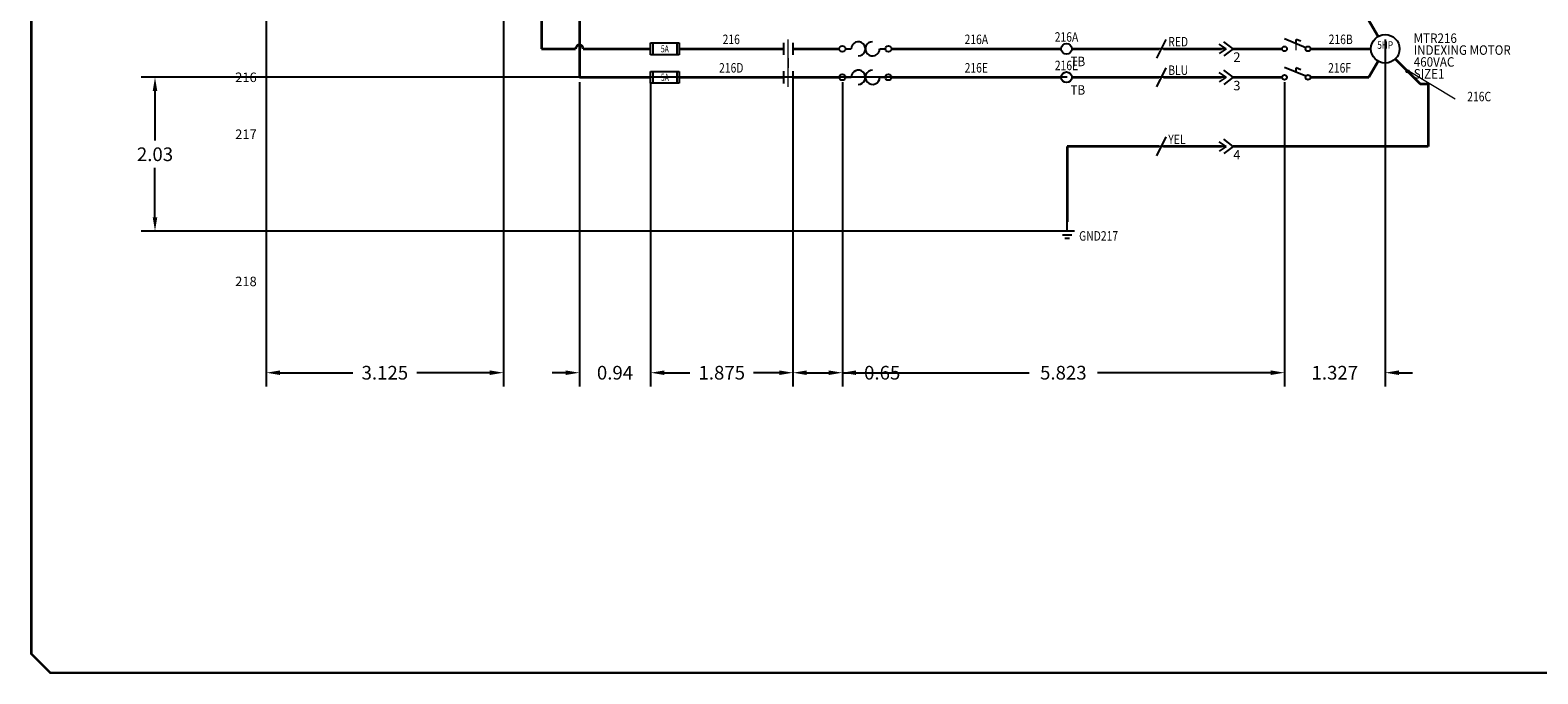
# Model space of a CAD drawing. Extents: x 0 to 33.5, y 0 to 22.4.
# Tile 1 of 8: x 0 to 19.9, y 0 to 8.5. Entities that reach past the tile are written whole.
import ezdxf
from ezdxf.enums import TextEntityAlignment as Align

# ---------------------------------------------------------------- set-up
doc = ezdxf.new("R2010")
doc.units = 0
doc.header["$MEASUREMENT"] = 0
for name, color, linetype, lineweight in [('A-ANNO-DIMS', 2, 'Continuous', 18), ('E-ANNO-TEXT', 3, 'Continuous', 18), ('LINK', 9, 'Continuous', 18), ('MISC', 7, 'Continuous', 13), ('SYMS', 7, 'Continuous', 25), ('TITLE', 7, 'Continuous', 35), ('WIRENO', 72, 'Continuous', 18), ('WIRES', 7, 'Continuous', 35)]:
    doc.layers.add(name, color=color, linetype=linetype, lineweight=lineweight)
for name, color, linetype in [('DESC', 150, 'Continuous'), ('TAGS', 150, 'Continuous'), ('TERMS', 123, 'Continuous'), ('WIREREF', 52, 'Continuous')]:
    doc.layers.add(name, color=color, linetype=linetype)
doc.styles.add('ITALIC', font='ITALIC')
doc.styles.add('SIMPLEX', font='SIMPLEX')
doc.styles.add('WD', font='romans.shx')
doc.dimstyles.get("Standard").update_dxf_attribs({"dimtxt": 0.18, "dimasz": 0.18, "dimexe": 0.18, "dimexo": 0.0625, "dimgap": 0.09, "dimtad": 0, "dimtih": 1, "dimtoh": 1, "dimdec": 4, "dimzin": 0, "dimdsep": 46, "dimtxsty": 'Standard', "dimcen": 0.09, "dimadec": 0, "dimazin": 0, "dimtfac": 1, "dimtdec": 4, "dimtofl": 0, "dimtmove": 0, "dimatfit": 3, "dimfxl": 1, "dimtolj": 1, "dimtzin": 0, "dimarcsym": 0})

# ---------------------------------------------------------------- blocks, each defined once
blk = doc.blocks.new('NO_NUM_acade_title')
at = {"layer": 'TITLE', "const_width": 0.0312}
blk.add_lwpolyline([(30.594, 0.281), (30.594, 22.177), (30.344, 22.427), (0.281, 22.427), (0.031, 22.177), (0.031, 0.281), (0.281, 0.031), (30.344, 0.031)], close=True, dxfattribs=at)
at = {"layer": 'TITLE', "style": 'ITALIC'}
for tag, height, p in [('TITLE#1', 0.125, (32.156, 3.406)), ('TITLE#2', 0.125, (32.156, 3.204)), ('TITLE#3', 0.125, (32.156, 3.001)), ('TITLE#4', 0.125, (32.156, 2.799)), ('DWG#', 0.2, (32.156, 0.826))]:
    blk.add_attdef(tag, text='', height=height, dxfattribs=at).set_placement(p, align=Align.CENTER)
at = {"layer": 'TITLE', "style": 'SIMPLEX'}
blk.add_attdef('CAD#', (30.826, 1.958), '', height=0.0938, rotation=90, dxfattribs=at)
at = {"layer": 'TITLE'}
for tag, p, height, style in [('JOB#', (31.464, 1.644), 0.0938, 'SIMPLEX'), ('SCALE', (31.353, 1.344), 0.0938, 'SIMPLEX'), ('DATE', (32.408, 1.344), 0.0938, 'SIMPLEX'), ('SHTS', (32.532, 0.25), 0.2, 'ITALIC')]:
    blk.add_attdef(tag, p, '', height=height, dxfattribs=dict(at, style=style))
at = {"layer": 'TITLE', "style": 'ITALIC'}
blk.add_attdef('SH#', text='', height=0.2, dxfattribs=at).set_placement((31.881, 0.25), align=Align.RIGHT)
at = {"layer": 'TITLE', "flags": 9}
blk.add_attdef('WD_TB', (31.219, 0.031), '', height=0.125, dxfattribs=at)
blk = doc.blocks.new('HFU1')
for p, q in [((-0.188, -0.078), (-0.188, 0.078)), ((-0.188, 0.078), (0.188, 0.078)), ((-0.156, 0.078), (-0.156, -0.078)), ((0.156, 0.078), (0.156, -0.078)), ((0.188, 0.078), (0.188, -0.078)), ((0.188, -0.078), (-0.188, -0.078))]:
    blk.add_line(p, q)
at = {"style": 'WD', "width": 0.7}
for tag, p in [('INST', (0, 0.422)), ('TAG1', (0, 0.125)), ('LOC', (0, 0.266))]:
    blk.add_attdef(tag, text='', height=0.125, dxfattribs=at).set_placement(p, align=Align.CENTER)
at = {"style": 'WD', "flags": 9}
for tag, p in [('ASSYCODE', (0.157, 0.251)), ('MFG', (0.156, 0.083)), ('CAT', (0.156, 0.102))]:
    blk.add_attdef(tag, text='', height=0.01, dxfattribs=at).set_placement(p, align=Align.CENTER)
at = {"style": 'WD'}
for tag, p, height, flags in [('X4TERM01', (-0.188, 0), 0.0109, 1), ('FAMILY', (0.129, 0.108), 0.01, 9), ('X1TERM02', (0.188, 0), 0.0109, 1)]:
    blk.add_attdef(tag, p, '', height=height, dxfattribs=dict(at, flags=flags))
at = {"style": 'WD', "width": 0.7}
blk.add_attdef('RATING1', text='', height=0.0938, dxfattribs=at).set_placement((0, 0), align=Align.MIDDLE_CENTER)
at = {"style": 'WD'}
for tag, p in [('X2LINK', (0, 0.109)), ('X8LINK', (0, -0.109))]:
    blk.add_attdef(tag, p, '', height=0.01, dxfattribs=at)
at = {"style": 'WD', "width": 0.7, "flags": 8}
blk.add_attdef('TERM01', text='', height=0.1, dxfattribs=at).set_placement((-0.25, -0.016), align=Align.TOP_RIGHT)
at = {"style": 'WD', "width": 0.7}
for tag, p in [('DESC1', (0.047, -0.234)), ('DESC2', (0.047, -0.391)), ('DESC3', (0.047, -0.547))]:
    blk.add_attdef(tag, text='', height=0.125, dxfattribs=at).set_placement(p, align=Align.MIDDLE_LEFT)
at = {"style": 'WD', "width": 0.7, "flags": 8}
blk.add_attdef('TERM02', text='', height=0.1, dxfattribs=at).set_placement((0.25, -0.016), align=Align.TOP_LEFT)
blk = doc.blocks.new('HCR21')
for p, q in [((-0.062, 0.08), (-0.062, -0.08)), ((0.062, 0.08), (0.062, -0.08))]:
    blk.add_line(p, q)
at = {"style": 'WD'}
for tag, width, p in [('INST', 0.7, (0, 0.451)), ('LOC', 0.7, (0, 0.281)), ('TAG2', 0.9, (0, 0.125)), ('XREF', 0.7, (0, -0.297)), ('DESC1', 0.7, (0, -0.449)), ('DESC2', 0.7, (0, -0.597)), ('DESC3', 0.7, (0, -0.744))]:
    blk.add_attdef(tag, text='', height=0.125, dxfattribs=dict(at, width=width)).set_placement(p, align=Align.CENTER)
for tag, p, height, flags in [('X4TERM01', (-0.062, 0), 0.0125, 1), ('X1TERM02', (0.062, 0), 0.0125, 1), ('CONTACT', (0.097, 0.036), 0.01, 1), ('FAMILY', (0.097, 0.053), 0.01, 9)]:
    blk.add_attdef(tag, p, '', height=height, dxfattribs=dict(at, flags=flags))
for tag, p in [('X2LINK', (0, 0.125)), ('X8LINK', (0, -0.125))]:
    blk.add_attdef(tag, p, '', height=0.01, dxfattribs=at)
at = {"style": 'WD', "flags": 8}
blk.add_attdef('TERM01', text='', height=0.125, dxfattribs=at).set_placement((-0.125, -0.016), align=Align.TOP_RIGHT)
blk.add_attdef('TERM02', text='', height=0.125, dxfattribs=at).set_placement((0.125, -0.016), align=Align.TOP_LEFT)
blk = doc.blocks.new('HOL1')
for p, q in [((-0.264, 0), (-0.188, 0)), ((0.188, 0), (0.264, 0))]:
    blk.add_line(p, q)
for centre in [(-0.304, 0), (0.304, 0)]:
    blk.add_circle(centre, 0.04)
for centre, start, end in [((-0.094, 0), 270.001, 180.002), ((0.094, 0), 90, 0.001)]:
    blk.add_arc(centre, 0.0938, start, end)
at = {"style": 'WD', "width": 0.7}
for tag, p in [('INST', (0, 0.795)), ('DESC1', (0, 0.469)), ('LOC', (0, 0.625)), ('DESC2', (0, 0.312)), ('RATING1', (0, -0.266))]:
    blk.add_attdef(tag, text='', height=0.125, dxfattribs=at).set_placement(p, align=Align.CENTER)
at = {"style": 'WD'}
blk.add_attdef('TAG1', text='', height=0.125, dxfattribs=at).set_placement((0, 0.156), align=Align.CENTER)
for tag, p, height, flags in [('X4TERM01', (-0.344, 0), 0.0125, 1), ('FAMILY', (0.205, 0.152), 0.01, 9), ('X1TERM02', (0.344, 0), 0.0125, 1)]:
    blk.add_attdef(tag, p, '', height=height, dxfattribs=dict(at, flags=flags))
for tag, p in [('X2LINK', (0, 0.125)), ('X8LINK', (0, -0.125))]:
    blk.add_attdef(tag, p, '', height=0.01, dxfattribs=at)
at = {"style": 'WD', "flags": 9}
for tag, p in [('ASSYCODE', (0.219, 0.062)), ('MFG', (0.228, 0.089)), ('CAT', (0.23, 0.108))]:
    blk.add_attdef(tag, text='', height=0.01, dxfattribs=at).set_placement(p, align=Align.CENTER)
at = {"style": 'WD', "flags": 8}
blk.add_attdef('TERM01', text='', height=0.125, dxfattribs=at).set_placement((-0.406, -0.031), align=Align.TOP_RIGHT)
blk.add_attdef('TERM02', text='', height=0.125, dxfattribs=at).set_placement((0.406, -0.031), align=Align.TOP_LEFT)
blk = doc.blocks.new('HT0W02')
blk.add_circle((0, 0), 0.0699)
at = {"style": 'WD'}
for tag, p, width in [('INST', (0.062, 0.42), 0.7), ('LOC', (0.062, 0.25), 0.7), ('DESC1', (0.053, -0.385), 0.8)]:
    blk.add_attdef(tag, p, '', height=0.125, dxfattribs=dict(at, width=width))
at = {"style": 'WD', "width": 0.8, "flags": 8}
blk.add_attdef('WIRENO', text='', height=0.125, dxfattribs=at).set_placement((0, 0.094), align=Align.CENTER)
at = {"style": 'WD', "flags": 1}
for tag, p, height in [('X4TERM01', (-0.07, 0), 0.0125), ('X4TERMDESC01', (-0.055, -0.023), 0.025), ('X2TERMDESC01', (-0.006, 0.029), 0.025), ('X2TERM01', (0, 0.07), 0.0125), ('STRIPSEQ', (0, 0), 0.00125), ('X1TERMDESC01', (0.039, -0.003), 0.025), ('X1TERM01', (0.07, 0), 0.0125), ('LINKTERM', (0, -0.002), 0.00125), ('X8TERM01', (0, -0.07), 0.0125), ('X8TERMDESC01', (0, -0.054), 0.025)]:
    blk.add_attdef(tag, p, '', height=height, dxfattribs=at)
at = {"style": 'WD'}
for tag, p, height, width, flags in [('TAGSTRIP', (0.053, -0.229), 0.125, 0.9, 8), ('ASSYCODE', (0.062, -0.281), 0.01, 0.7, 1), ('CAT', (0.213, -0.406), 0.109, 0.8, 1), ('DESC2', (0.053, -0.541), 0.125, 0.8, 8), ('DESC3', (0.053, -0.698), 0.125, 0.8, 8)]:
    blk.add_attdef(tag, p, '', height=height, dxfattribs=dict(at, width=width, flags=flags))
at = {"style": 'WD', "width": 0.8, "flags": 1}
blk.add_attdef('MFG', text='', height=0.109, dxfattribs=at).set_placement((0.088, -0.406), align=Align.RIGHT)
blk = doc.blocks.new('HDS11')
for p, q in [((0.126, 0.013), (-0.156, 0.13)), ((0, 0.065), (0, 0.125)), ((0.062, 0.099), (0, 0.125))]:
    blk.add_line(p, q)
for centre in [(-0.155, 0), (0.155, 0)]:
    blk.add_circle(centre, 0.0322)
at = {"style": 'WD', "width": 0.7}
for tag, p in [('INST', (0, 0.625)), ('LOC', (0, 0.469)), ('RATING1', (0, 0.156)), ('XREF', (0, -0.236)), ('DESC1', (0, -0.406)), ('DESC2', (0, -0.562))]:
    blk.add_attdef(tag, text='', height=0.125, dxfattribs=at).set_placement(p, align=Align.CENTER)
at = {"style": 'WD'}
blk.add_attdef('TAG1', text='', height=0.125, dxfattribs=at).set_placement((0, 0.312), align=Align.CENTER)
for tag, p in [('X2LINK', (0, 0.438)), ('X8LINK', (0, -0.016))]:
    blk.add_attdef(tag, p, '', height=0.01, dxfattribs=at)
for tag, p, height, flags in [('X4TERM01', (-0.188, 0), 0.0125, 1), ('X1TERM02', (0.188, 0), 0.0125, 1), ('CONTACT', (0.206, 0.04), 0.01, 9), ('FAMILY', (0.206, 0.131), 0.01, 9)]:
    blk.add_attdef(tag, p, '', height=height, dxfattribs=dict(at, flags=flags))
at = {"style": 'WD', "flags": 9}
for tag, p in [('ASSYCODE', (0.219, 0.062)), ('MFG', (0.228, 0.089)), ('CAT', (0.23, 0.108))]:
    blk.add_attdef(tag, text='', height=0.01, dxfattribs=at).set_placement(p, align=Align.CENTER)
at = {"style": 'WD', "flags": 8}
blk.add_attdef('TERM01', text='', height=0.125, dxfattribs=at).set_placement((-0.25, -0.031), align=Align.TOP_RIGHT)
blk.add_attdef('TERM02', text='', height=0.125, dxfattribs=at).set_placement((0.25, -0.031), align=Align.TOP_LEFT)
blk = doc.blocks.new('HMO13')
blk.add_circle((0, 0), 0.188)
at = {"style": 'WD'}
for tag, p, width in [('INST', (0.381, 0.403), 0.7), ('TAG1', (0.375, 0.077), 0.9), ('LOC', (0.381, 0.234), 0.7), ('DESC1', (0.376, -0.079), 0.9), ('DESC2', (0.376, -0.235), 0.9), ('DESC3', (0.376, -0.391), 0.9), ('RATING3', (0.375, -0.548), 0.8), ('RATING4', (0.375, -0.704), 0.8), ('WDTAGALT', (0.375, -0.875), 0.7)]:
    blk.add_attdef(tag, p, '', height=0.125, dxfattribs=dict(at, width=width))
at = {"style": 'WD', "width": 0.8}
blk.add_attdef('RATING1', text='', height=0.1, dxfattribs=at).set_placement((0, 0), align=Align.CENTER)
at = {"style": 'WD', "flags": 1}
for tag, p in [('X4TERM02', (-0.188, 0)), ('X0TERM01', (-0.094, 0.162)), ('X0TERM03', (-0.094, -0.162)), ('X0TERM04', (0.133, -0.133))]:
    blk.add_attdef(tag, p, '', height=0.0125, dxfattribs=at)
at = {"style": 'WD', "flags": 9}
for tag, p in [('ASSYCODE', (0, 0.125)), ('FAMILY', (-0.005, 0.17))]:
    blk.add_attdef(tag, text='', height=0.01, dxfattribs=at).set_placement(p, align=Align.CENTER)
at = {"style": 'WD', "flags": 1}
for tag, p in [('MFG', (0, 0.14)), ('CAT', (0, 0.159))]:
    blk.add_attdef(tag, text='', height=0.01, dxfattribs=at).set_placement(p, align=Align.MIDDLE)
at = {"style": 'WD', "width": 0.8}
blk.add_attdef('RATING2', text='', height=0.1, dxfattribs=at).set_placement((0, -0.031), align=Align.TOP_CENTER)
blk = doc.blocks.new('VGND2')
for p, q in [((0, -0.125), (0, 0)), ((0.09375, -0.125), (-0.09375, -0.125)), ((-0.0625, -0.171875), (0.0625, -0.171875)), ((-0.03125, -0.21875), (0.03125, -0.21875))]:
    blk.add_line(p, q)
at = {"style": 'WD', "flags": 1}
for tag in ['ASSYCODE', 'X2TERM01', 'CAT', 'MFG', 'FAMILY']:
    blk.add_attdef(tag, (0, 0), '', height=0.01, dxfattribs=at)
at = {"style": 'WD', "width": 0.8}
for tag, p in [('INST', (0.15625, 0.125)), ('LOC', (0.15625, -0.03125)), ('TAG1', (0.15625, -0.1875)), ('DESC1', (0.15625, -0.34375)), ('DESC2', (0.15625, -0.5))]:
    blk.add_attdef(tag, text='', height=0.125, dxfattribs=at).set_placement(p, align=Align.MIDDLE_LEFT)
blk = doc.blocks.new('HCN2PJ')
for p, q in [((-0.031, 0), (-0.125, 0.062)), ((-0.031, 0), (-0.125, -0.062)), ((-0.031, 0), (-0.094, 0)), ((0.062, 0), (-0.062, 0.094)), ((0.062, 0), (-0.062, -0.094))]:
    blk.add_line(p, q)
at = {"style": 'WD', "width": 0.7}
for tag, p in [('DESC1', (-0.031, 0.406)), ('DESC2', (-0.031, 0.25))]:
    blk.add_attdef(tag, text='', height=0.125, dxfattribs=at).set_placement(p, align=Align.RIGHT)
for tag, p in [('INST', (0.094, 0.406)), ('LOC', (0.094, 0.25))]:
    blk.add_attdef(tag, p, '', height=0.125, dxfattribs=at)
at = {"style": 'WD'}
for tag, p, height in [('TAG2', (0.094, 0.094), 0.125), ('X2LINK', (-0.062, 0.125), 0.01), ('X8LINK', (-0.062, -0.125), 0.01)]:
    blk.add_attdef(tag, p, '', height=height, dxfattribs=at)
for tag, p, height, flags in [('X4TERMDESC01', (-0.113, 0.019), 0.01, 1), ('X4TERM01', (-0.094, 0), 0.0125, 1), ('FAMILY', (0.048, 0.121), 0.01, 9), ('X1TERM02', (0.062, 0), 0.0125, 1), ('X1TERMDESC02', (0.067, 0.014), 0.01, 1)]:
    blk.add_attdef(tag, p, '', height=height, dxfattribs=dict(at, flags=flags))
at = {"style": 'WD', "flags": 8}
blk.add_attdef('TERM01', text='', height=0.125, dxfattribs=at).set_placement((-0.156, -0.047), align=Align.TOP_RIGHT)
blk.add_attdef('TERM02', text='', height=0.125, dxfattribs=at).set_placement((0.062, -0.047), align=Align.TOP_LEFT)
blk = doc.blocks.new('HW02')
for p, q in [((0.062, 0.125), (-0.062, -0.125)), ((0.031, 0), (-0.031, 0))]:
    blk.add_line(p, q)
at = {"style": 'WD', "width": 0.7, "flags": 1}
for tag, p in [('INST', (0, 0.357)), ('LOC', (0, 0.188)), ('XREF', (0, -0.3)), ('DESC1', (0, -0.456)), ('DESC2', (0, -0.613))]:
    blk.add_attdef(tag, text='', height=0.125, dxfattribs=at).set_placement(p, align=Align.CENTER)
at = {"style": 'WD', "width": 0.8}
blk.add_attdef('TAG2', text='', height=0.125, dxfattribs=at).set_placement((-0.031, 0.031), align=Align.RIGHT)
at = {"style": 'WD', "flags": 1}
for tag, p in [('X4TERM01', (-0.031, 0)), ('X1TERM01', (0.031, 0))]:
    blk.add_attdef(tag, p, '', height=0.0125, dxfattribs=at)
at = {"style": 'WD'}
for tag, p in [('X2LINK', (0, 0.125)), ('X8LINK', (0, -0.125))]:
    blk.add_attdef(tag, p, '', height=0.01, dxfattribs=at)
at = {"style": 'WD', "flags": 9}
blk.add_attdef('FAMILY', text='', height=0.01, dxfattribs=at).set_placement((0.023, 0.118), align=Align.CENTER)
at = {"style": 'WD', "width": 0.8}
blk.add_attdef('RATING1', (0.094, 0.031), '', height=0.125, dxfattribs=at)
blk = doc.blocks.new('WD_WNH')
at = {"style": 'WD', "width": 0.8}
blk.add_attdef('WIRENO', text='', height=0.125, dxfattribs=at).set_placement((0, 0.062), align=Align.CENTER)
at = {"style": 'WD', "flags": 1}
for tag, p in [('W01USER', (0, 0.078)), ('W02USER', (0, 0.07)), ('W03USER', (0, 0.062)), ('W04USER', (0, 0.055)), ('W05USER', (0, 0.047)), ('W06USER', (0, 0.039)), ('W07USER', (0, 0.031)), ('W08USER', (0, 0.023)), ('W09USER', (0, 0.016)), ('W10USER', (0, 0.008))]:
    blk.add_attdef(tag, text='', height=0.005, dxfattribs=at).set_placement(p, align=Align.CENTER)
blk = doc.blocks.new('*D36')
at = {"layer": 'A-ANNO-DIMS', "color": 0, "lineweight": -2, "transparency": 16777216}
for p, q in [((3.125, 17.5625), (3.125, 3.802917)), ((6.25, 17.5625), (6.25, 3.802917)), ((3.305, 3.982917), (4.2675, 3.982917)), ((6.07, 3.982917), (5.1075, 3.982917))]:
    blk.add_line(p, q, dxfattribs=at)
at = {"layer": 'A-ANNO-DIMS', "color": 0, "transparency": 16777216}
for points in [[(3.305, 4.012917), (3.305, 3.952917), (3.125, 3.982917)], [(6.07, 4.012917), (6.07, 3.952917), (6.25, 3.982917)]]:
    blk.add_solid(points, dxfattribs=at)
at = {"layer": 'Defpoints', "color": 0, "transparency": 16777216}
for p in [(3.125, 17.625), (6.25, 17.625), (6.25, 3.982917)]:
    blk.add_point(p, dxfattribs=at)
at = {"layer": 'A-ANNO-DIMS', "color": 0, "transparency": 16777216, "insert": (4.6875, 3.982917), "char_height": 0.18, "attachment_point": 5}
blk.add_mtext('\\A1;3.125', dxfattribs=at)
blk = doc.blocks.new('*D41')
at = {"layer": 'A-ANNO-DIMS', "color": 0, "lineweight": -2, "transparency": 16777216}
for p, q in [((7.25, 7.8125), (7.25, 3.802917)), ((8.1875, 7.8125), (8.1875, 3.802917)), ((7.07, 3.982917), (6.89, 3.982917)), ((8.3675, 3.982917), (8.5475, 3.982917))]:
    blk.add_line(p, q, dxfattribs=at)
at = {"layer": 'A-ANNO-DIMS', "color": 0, "transparency": 16777216}
for points in [[(7.07, 4.012917), (7.07, 3.952917), (7.25, 3.982917)], [(8.3675, 4.012917), (8.3675, 3.952917), (8.1875, 3.982917)]]:
    blk.add_solid(points, dxfattribs=at)
at = {"layer": 'Defpoints', "color": 0, "transparency": 16777216}
for p in [(7.25, 7.875), (8.1875, 7.875), (8.1875, 3.982917)]:
    blk.add_point(p, dxfattribs=at)
at = {"layer": 'A-ANNO-DIMS', "color": 0, "transparency": 16777216, "insert": (7.71875, 3.982917), "char_height": 0.18, "attachment_point": 5}
blk.add_mtext('\\A1;0.94', dxfattribs=at)
blk = doc.blocks.new('*D42')
at = {"layer": 'A-ANNO-DIMS', "color": 0, "lineweight": -2, "transparency": 16777216}
for p, q in [((8.1875, 7.8125), (8.1875, 3.802917)), ((10.0625, 7.8125), (10.0625, 3.802917)), ((8.3675, 3.982917), (8.705, 3.982917)), ((9.8825, 3.982917), (9.545, 3.982917))]:
    blk.add_line(p, q, dxfattribs=at)
at = {"layer": 'A-ANNO-DIMS', "color": 0, "transparency": 16777216}
for points in [[(8.3675, 4.012917), (8.3675, 3.952917), (8.1875, 3.982917)], [(9.8825, 4.012917), (9.8825, 3.952917), (10.0625, 3.982917)]]:
    blk.add_solid(points, dxfattribs=at)
at = {"layer": 'Defpoints', "color": 0, "transparency": 16777216}
for p in [(8.1875, 7.875), (10.0625, 7.875), (10.0625, 3.982917)]:
    blk.add_point(p, dxfattribs=at)
at = {"layer": 'A-ANNO-DIMS', "color": 0, "transparency": 16777216, "insert": (9.125, 3.982917), "char_height": 0.18, "attachment_point": 5}
blk.add_mtext('\\A1;1.875', dxfattribs=at)
blk = doc.blocks.new('*D43')
at = {"layer": 'A-ANNO-DIMS', "color": 0, "lineweight": -2, "transparency": 16777216}
for p, q in [((10.0625, 7.8125), (10.0625, 3.802917)), ((10.712955, 7.8125), (10.712955, 3.802917)), ((10.2425, 3.982917), (10.532955, 3.982917)), ((10.712955, 3.982917), (10.892955, 3.982917))]:
    blk.add_line(p, q, dxfattribs=at)
at = {"layer": 'A-ANNO-DIMS', "color": 0, "transparency": 16777216}
for points in [[(10.2425, 4.012917), (10.2425, 3.952917), (10.0625, 3.982917)], [(10.532955, 4.012917), (10.532955, 3.952917), (10.712955, 3.982917)]]:
    blk.add_solid(points, dxfattribs=at)
at = {"layer": 'Defpoints', "color": 0, "transparency": 16777216}
for p in [(10.0625, 7.875), (10.712955, 7.875), (10.712955, 3.982917)]:
    blk.add_point(p, dxfattribs=at)
at = {"layer": 'A-ANNO-DIMS', "color": 0, "transparency": 16777216, "insert": (11.237955, 3.982917), "char_height": 0.18, "attachment_point": 5}
blk.add_mtext('\\A1;0.65', dxfattribs=at)
blk = doc.blocks.new('*D44')
at = {"layer": 'A-ANNO-DIMS', "color": 0, "lineweight": -2, "transparency": 16777216}
for p, q in [((10.713, 7.812), (10.713, 3.803)), ((16.536, 7.812), (16.536, 3.803)), ((10.893, 3.983), (13.174, 3.983)), ((16.356, 3.983), (14.074, 3.983))]:
    blk.add_line(p, q, dxfattribs=at)
at = {"layer": 'A-ANNO-DIMS', "color": 0, "transparency": 16777216}
for points in [[(10.893, 4.013), (10.893, 3.953), (10.713, 3.983)], [(16.356, 4.013), (16.356, 3.953), (16.536, 3.983)]]:
    blk.add_solid(points, dxfattribs=at)
at = {"layer": 'Defpoints', "color": 0, "transparency": 16777216}
for p in [(10.713, 7.875), (16.536, 7.875), (16.536, 3.983)]:
    blk.add_point(p, dxfattribs=at)
at = {"layer": 'A-ANNO-DIMS', "color": 0, "transparency": 16777216, "insert": (13.624, 3.983), "char_height": 0.18, "attachment_point": 5}
blk.add_mtext('\\A1;5.823', dxfattribs=at)
blk = doc.blocks.new('*D45')
at = {"layer": 'A-ANNO-DIMS', "color": 0, "lineweight": -2, "transparency": 16777216}
for p, q in [((17.862828, 8.375), (17.862828, 3.802917)), ((16.53586, 7.8125), (16.53586, 3.802917)), ((16.35586, 3.982917), (16.17586, 3.982917)), ((18.042828, 3.982917), (18.222828, 3.982917))]:
    blk.add_line(p, q, dxfattribs=at)
at = {"layer": 'A-ANNO-DIMS', "color": 0, "transparency": 16777216}
for points in [[(16.35586, 4.012917), (16.35586, 3.952917), (16.53586, 3.982917)], [(18.042828, 4.012917), (18.042828, 3.952917), (17.862828, 3.982917)]]:
    blk.add_solid(points, dxfattribs=at)
at = {"layer": 'Defpoints', "color": 0, "transparency": 16777216}
for p in [(17.862828, 8.4375), (16.53586, 7.875), (17.862828, 3.982917)]:
    blk.add_point(p, dxfattribs=at)
at = {"layer": 'A-ANNO-DIMS', "color": 0, "transparency": 16777216, "insert": (17.199344, 3.982917), "char_height": 0.18, "attachment_point": 5}
blk.add_mtext('\\A1;1.327', dxfattribs=at)
blk = doc.blocks.new('*D48')
at = {"layer": 'A-ANNO-DIMS', "color": 0, "lineweight": -2, "transparency": 16777216}
for p, q in [((13.673, 7.875), (1.48, 7.875)), ((1.66, 7.695), (1.66, 7.041)), ((1.66, 6.028), (1.66, 6.681)), ((13.613, 5.848), (1.48, 5.848))]:
    blk.add_line(p, q, dxfattribs=at)
at = {"layer": 'A-ANNO-DIMS', "color": 0, "transparency": 16777216}
for points in [[(1.63, 7.695), (1.69, 7.695), (1.66, 7.875)], [(1.63, 6.028), (1.69, 6.028), (1.66, 5.848)]]:
    blk.add_solid(points, dxfattribs=at)
at = {"layer": 'Defpoints', "color": 0, "transparency": 16777216}
for p in [(13.735, 7.875), (1.66, 5.848), (13.675, 5.848)]:
    blk.add_point(p, dxfattribs=at)
at = {"layer": 'A-ANNO-DIMS', "color": 0, "transparency": 16777216, "insert": (1.66, 6.861), "char_height": 0.18, "attachment_point": 5}
blk.add_mtext('\\A1;2.03', dxfattribs=at)

msp = doc.modelspace()

# ---------------------------------------------------------------- linework, layer by layer
at = {"layer": 'LINK'}
for points in [[(10, 7.75), (10, 8.375)], [(16.6912, 8.2344), (16.6912, 8.3125)], [(10, 8.125), (10, 8)]]:
    msp.add_lwpolyline(points, dxfattribs=at)
at = {"layer": 'WIRENO'}
msp.add_lwpolyline([(18.7839, 7.5846), (18.1889, 7.9463), (18.1777, 7.9654), (18.1475, 7.9732), (18.1284, 7.962), (18.1396, 7.943), (18.1699, 7.9351), (18.1794, 7.9407)], dxfattribs=at)
at = {"layer": 'WIRES'}
for p, q in [((6.75, 17.575), (6.75, 8.25)), ((7.25, 17.625), (7.25, 7.875)), ((17.5742, 8.75), (17.7691, 8.4124)), ((6.75, 8.25), (7.2, 8.25)), ((7.3, 8.25), (8.1875, 8.25)), ((8.5625, 8.25), (9.9375, 8.25)), ((10.0625, 8.25), (10.673, 8.25)), ((11.3605, 8.25), (13.5956, 8.25)), ((13.7353, 8.25), (14.8807, 8.25)), ((14.9432, 8.25), (15.7062, 8.25)), ((15.8625, 8.25), (16.5036, 8.25)), ((16.8786, 8.25), (17.6753, 8.25)), ((17.6463, 7.875), (17.7691, 8.0876)), ((17.9954, 8.1174), (18.3219, 7.7909)), ((7.25, 7.875), (8.1875, 7.875)), ((8.5625, 7.875), (9.9375, 7.875)), ((10.0625, 7.875), (10.673, 7.875)), ((11.3605, 7.875), (13.5956, 7.875)), ((13.7353, 7.875), (14.8807, 7.875)), ((14.9432, 7.875), (15.7062, 7.875)), ((15.8625, 7.875), (16.5036, 7.875)), ((16.8786, 7.875), (17.6463, 7.875)), ((18.3219, 7.7909), (18.4284, 7.7909)), ((18.4284, 7.7909), (18.4284, 6.9643)), ((13.6752, 6.9643), (13.6752, 5.9728)), ((14.8807, 6.9643), (13.6752, 6.9643)), ((15.7062, 6.9643), (14.9432, 6.9643)), ((18.4284, 6.9643), (15.8625, 6.9643))]:
    msp.add_line(p, q, dxfattribs=at)
msp.add_arc((7.25, 8.25), 0.05, 0, 180, dxfattribs=at)

# ---------------------------------------------------------------- block references
at = {"layer": 'SYMS'}
for name, p in [('HOL1', (11.0167, 8.25)), ('HDS11', (16.6911, 8.25)), ('HCR21', (10, 8.25)), ('HCR21', (10, 7.875)), ('HOL1', (11.0167, 7.875)), ('HDS11', (16.6911, 7.875))]:
    msp.add_blockref(name, p, dxfattribs=at)
ref = msp.add_blockref('HT0W02', (13.6654, 8.25), dxfattribs=at)
ref.add_attrib('WIRENO', '216A', dxfattribs={"layer": 'WIREREF', "linetype": 'Continuous', "height": 0.125, "style": 'WD', "width": 0.8, "flags": 8}).set_placement((13.6654, 8.3437), align=Align.CENTER)
ref.add_attrib('TAGSTRIP', 'TB', (13.7186, 8.0212), dxfattribs={"layer": 'TAGS', "linetype": 'Continuous', "height": 0.125, "style": 'WD', "width": 0.9, "flags": 8})
ref = msp.add_blockref('HW02', (14.912, 8.25), dxfattribs=at)
ref.add_attrib('RATING1', 'RED', (15.0057, 8.2812), dxfattribs={"layer": 'MISC', "height": 0.125, "style": 'WD', "width": 0.8})
ref = msp.add_blockref('HCN2PJ', (15.8, 8.25), dxfattribs=at)
ref.add_attrib('TERM02', '2', dxfattribs={"layer": 'TERMS', "linetype": 'Continuous', "height": 0.125, "style": 'WD', "flags": 8}).set_placement((15.8625, 8.203), align=Align.TOP_LEFT)
ref = msp.add_blockref('HMO13', (17.8628, 8.25), dxfattribs=at)
ref.add_attrib('DESC3', 'SIZE1', (18.2389, 7.8586), dxfattribs={"layer": 'DESC', "height": 0.125, "style": 'WD', "width": 0.9})
ref.add_attrib('RATING1', '5HP', dxfattribs={"layer": 'MISC', "height": 0.1, "style": 'WD', "width": 0.8}).set_placement((17.8628, 8.25), align=Align.CENTER)
ref.add_attrib('DESC1', 'INDEXING MOTOR', (18.2389, 8.1711), dxfattribs={"layer": 'DESC', "height": 0.125, "style": 'WD', "width": 0.9})
ref.add_attrib('DESC2', '460VAC', (18.2389, 8.0149), dxfattribs={"layer": 'DESC', "height": 0.125, "style": 'WD', "width": 0.9})
ref.add_attrib('TAG1', 'MTR216', (18.2378, 8.3274), dxfattribs={"layer": 'TAGS', "height": 0.125, "style": 'WD', "width": 0.9})
ref = msp.add_blockref('HFU1', (8.375, 8.25), dxfattribs=at)
ref.add_attrib('RATING1', '5A', dxfattribs={"layer": 'MISC', "height": 0.09375, "style": 'WD', "width": 0.7}).set_placement((8.375, 8.25), align=Align.MIDDLE_CENTER)
ref = msp.add_blockref('HFU1', (8.375, 7.875), dxfattribs=at)
ref.add_attrib('RATING1', '5A', dxfattribs={"layer": 'MISC', "height": 0.09375, "style": 'WD', "width": 0.7}).set_placement((8.375, 7.875), align=Align.MIDDLE_CENTER)
ref = msp.add_blockref('HT0W02', (13.6654, 7.875), dxfattribs=at)
ref.add_attrib('WIRENO', '216E', dxfattribs={"layer": 'WIREREF', "linetype": 'Continuous', "height": 0.125, "style": 'WD', "width": 0.8, "flags": 8}).set_placement((13.6654, 7.9688), align=Align.CENTER)
ref.add_attrib('TAGSTRIP', 'TB', (13.7186, 7.6462), dxfattribs={"layer": 'TAGS', "linetype": 'Continuous', "height": 0.125, "style": 'WD', "width": 0.9, "flags": 8})
ref = msp.add_blockref('HW02', (14.912, 7.875), dxfattribs=at)
ref.add_attrib('RATING1', 'BLU', (15.0057, 7.9062), dxfattribs={"layer": 'MISC', "height": 0.125, "style": 'WD', "width": 0.8})
ref = msp.add_blockref('HCN2PJ', (15.8, 7.875), dxfattribs=at)
ref.add_attrib('TERM02', '3', dxfattribs={"layer": 'TERMS', "linetype": 'Continuous', "height": 0.125, "style": 'WD', "flags": 8}).set_placement((15.8625, 7.828), align=Align.TOP_LEFT)
ref = msp.add_blockref('HW02', (14.912, 6.9643), dxfattribs=at)
ref.add_attrib('RATING1', 'YEL', (15.0057, 6.9955), dxfattribs={"layer": 'MISC', "height": 0.125, "style": 'WD', "width": 0.8})
ref = msp.add_blockref('HCN2PJ', (15.8, 6.9643), dxfattribs=at)
ref.add_attrib('TERM02', '4', dxfattribs={"layer": 'TERMS', "linetype": 'Continuous', "height": 0.125, "style": 'WD', "flags": 8}).set_placement((15.8625, 6.9173), align=Align.TOP_LEFT)
ref = msp.add_blockref('VGND2', (13.6752, 5.9728), dxfattribs=at)
ref.add_attrib('TAG1', 'GND217', dxfattribs={"layer": 'TAGS', "height": 0.125, "style": 'WD', "width": 0.8}).set_placement((13.8315, 5.7853), align=Align.MIDDLE_LEFT)
at = {"layer": 'TITLE'}
msp.add_blockref('NO_NUM_acade_title', (0, 0), dxfattribs=at)
at = {"layer": 'WIRENO'}
ref = msp.add_blockref('WD_WNH', (9.25, 8.25), dxfattribs=at)
ref.add_attrib('WIRENO', '216', dxfattribs={"linetype": 'Continuous', "height": 0.125, "style": 'WD', "width": 0.8}).set_placement((9.25, 8.3125), align=Align.CENTER)
ref = msp.add_blockref('WD_WNH', (12.478, 8.25), dxfattribs=at)
ref.add_attrib('WIRENO', '216A', dxfattribs={"linetype": 'Continuous', "height": 0.125, "style": 'WD', "width": 0.8}).set_placement((12.478, 8.3125), align=Align.CENTER)
ref = msp.add_blockref('WD_WNH', (17.277, 8.25), dxfattribs=at)
ref.add_attrib('WIRENO', '216B', dxfattribs={"linetype": 'Continuous', "height": 0.125, "style": 'WD', "width": 0.8}).set_placement((17.277, 8.3125), align=Align.CENTER)
ref = msp.add_blockref('WD_WNH', (9.25, 7.875), dxfattribs=at)
ref.add_attrib('WIRENO', '216D', dxfattribs={"linetype": 'Continuous', "height": 0.125, "style": 'WD', "width": 0.8}).set_placement((9.25, 7.9375), align=Align.CENTER)
ref = msp.add_blockref('WD_WNH', (12.478, 7.875), dxfattribs=at)
ref.add_attrib('WIRENO', '216E', dxfattribs={"linetype": 'Continuous', "height": 0.125, "style": 'WD', "width": 0.8}).set_placement((12.478, 7.9375), align=Align.CENTER)
ref = msp.add_blockref('WD_WNH', (17.2625, 7.875), dxfattribs=at)
ref.add_attrib('WIRENO', '216F', dxfattribs={"linetype": 'Continuous', "height": 0.125, "style": 'WD', "width": 0.8}).set_placement((17.2625, 7.9375), align=Align.CENTER)
ref = msp.add_blockref('WD_WNH', (18.1587, 7.9542), dxfattribs=at)
ref.add_attrib('WIRENO', '216C', dxfattribs={"linetype": 'Continuous', "height": 0.125, "style": 'WD', "width": 0.8}).set_placement((19.1007, 7.6836), align=Align.TOP_CENTER)

# ---------------------------------------------------------------- texts
at = {"layer": 'E-ANNO-TEXT', "style": 'WD'}
for s, p in [('216', (3, 7.875)), ('217', (3, 7.125)), ('218', (3, 5.1858))]:
    msp.add_text(s, height=0.125, dxfattribs=at).set_placement(p, align=Align.MIDDLE_RIGHT)

# ---------------------------------------------------------------- dimensions: what is measured, and where the dimension line sits
at = {"layer": 'A-ANNO-DIMS'}
for base, p1, p2, override, picture, middle in [((6.25, 3.9829), (3.125, 17.625), (6.25, 17.625), {"dimdec": 3, "dimlfac": 1, "dimrnd": 0, "dimzin": 0, "dimdsep": 46, "dimlunit": 2}, '*D36', (4.6875, 3.9829)), ((17.8628, 3.9829), (16.5359, 7.875), (17.8628, 8.4375), {"dimdec": 3, "dimlfac": 1, "dimrnd": 0, "dimzin": 0, "dimdsep": 46, "dimlunit": 2}, '*D45', (17.1993, 3.9829)), ((8.1875, 3.9829), (7.25, 7.875), (8.1875, 7.875), {"dimdec": 2, "dimlfac": 1, "dimrnd": 0, "dimzin": 0, "dimdsep": 46, "dimlunit": 2}, '*D41', (7.7188, 3.9829)), ((10.0625, 3.9829), (8.1875, 7.875), (10.0625, 7.875), {"dimdec": 3, "dimlfac": 1, "dimrnd": 0, "dimzin": 0, "dimdsep": 46, "dimlunit": 2}, '*D42', (9.125, 3.9829)), ((10.713, 3.9829), (10.0625, 7.875), (10.713, 7.875), {"dimdec": 2, "dimlfac": 1, "dimrnd": 0, "dimzin": 0, "dimdsep": 46, "dimlunit": 2}, '*D43', (11.238, 3.9829)), ((16.5359, 3.9829), (10.713, 7.875), (16.5359, 7.875), {"dimdec": 3, "dimlfac": 1, "dimrnd": 0, "dimzin": 0, "dimdsep": 46, "dimlunit": 2}, '*D44', (13.6244, 3.9829))]:
    dim = msp.add_linear_dim(base=base, p1=p1, p2=p2, dimstyle='Standard', override=override, dxfattribs=at)
    dim.commit()
    dim.dimension.update_dxf_attribs({"geometry": picture, "text_midpoint": middle})
dim = msp.add_linear_dim(base=(1.66, 5.8478), p1=(13.7353, 7.875), p2=(13.6752, 5.8478), angle=90, dimstyle='Standard', override={"dimdec": 2, "dimlfac": 1, "dimrnd": 0, "dimzin": 0, "dimdsep": 46, "dimlunit": 2}, dxfattribs=at)
dim.commit()
dim.dimension.update_dxf_attribs({"geometry": '*D48', "text_midpoint": (1.66, 6.8614)})

doc.saveas('drawing.dxf')
